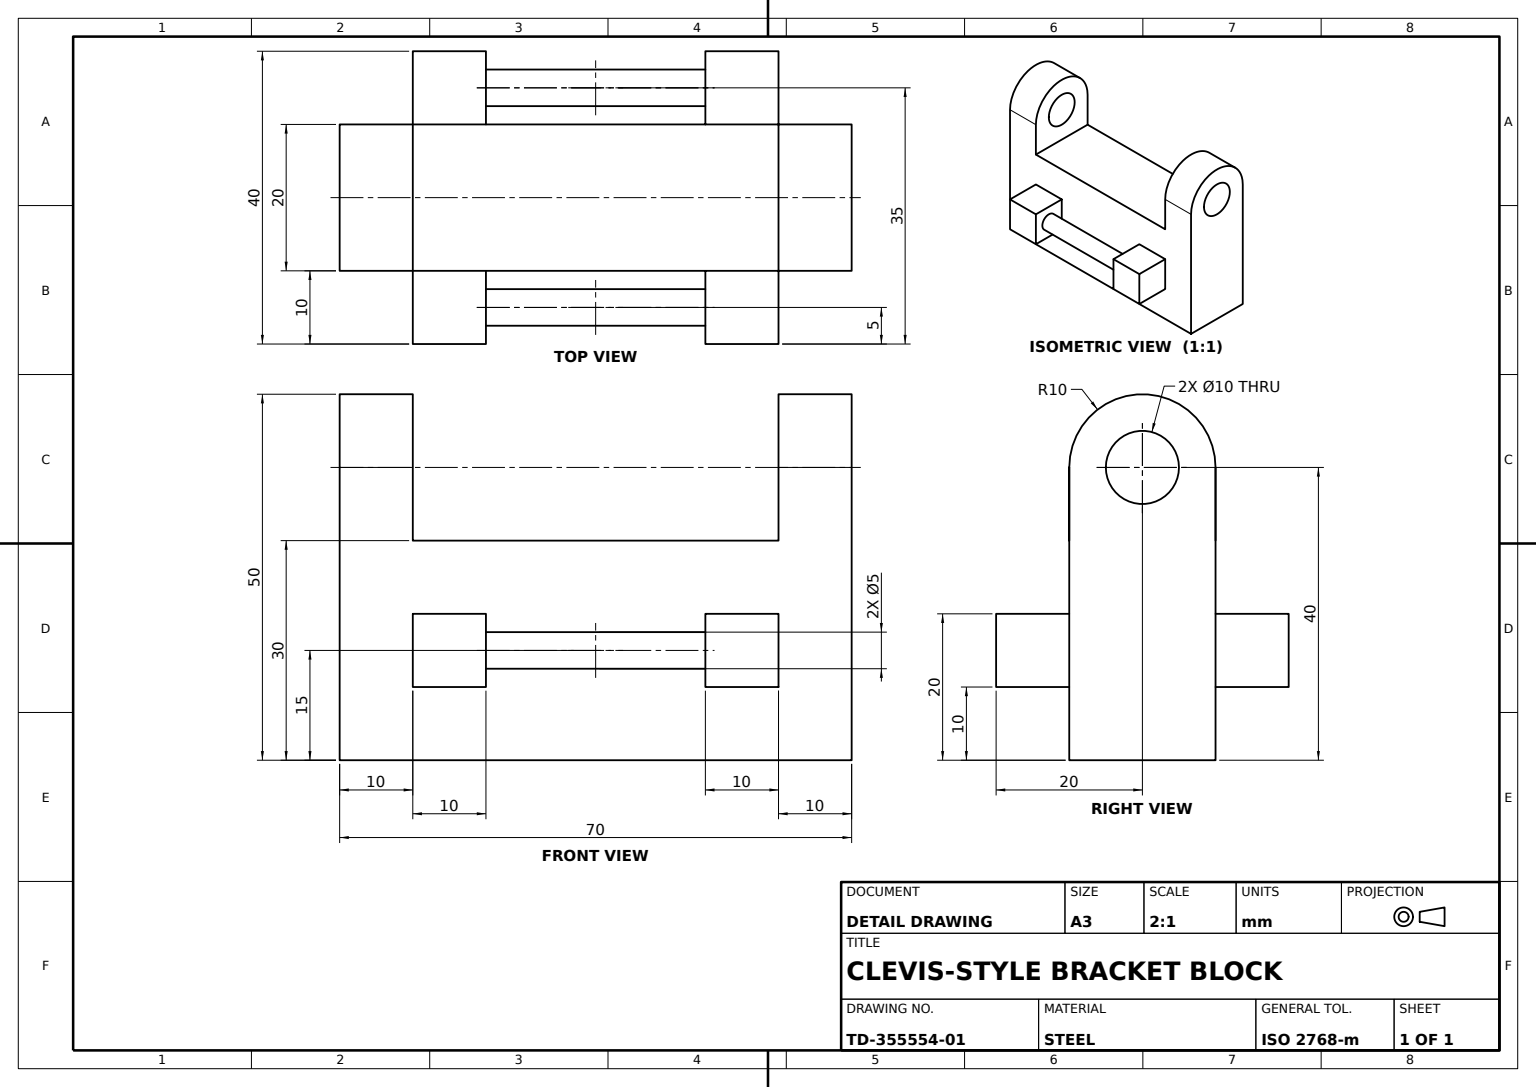
SolidWorks part; units mm, degrees
material "Plain Carbon Steel"
ref_plane "Front Plane" through (0, 0, 0) normal (0, 0, 1) x (1, 0, 0)
ref_plane "Top Plane" through (0, 0, 0) normal (0, 1, 0) x (1, 0, 0)
ref_plane "Right Plane" through (0, 0, 0) normal (1, 0, 0) x (0, 0, -1)
sketch "Base Block Sketch" plane through (0, 0, 0) normal (0, 0, 1) x (1, 0, 0)
  line L0 (0, 0) -> (70, 0)
  line L1 (70, 0) -> (70, 30)
  line L2 (70, 30) -> (0, 30)
  line L3 (0, 30) -> (0, 0)
  dimension "D1" = 70
  dimension "D2" = 30
extrude "Base Block" add sketch "Base Block Sketch" along normal blind 20
ref_plane "Hinge Ear Sketch Plane" through (0, 0, 0) normal (1, 0, 0) x (0, 0, -1)
sketch "Hinge Ear Sketch" plane through (0, 0, 0) normal (1, 0, 0) x (0, 0, -1)
  line L0 (-20, 30) -> (0, 30) construction
  line L1 (-20, 40) -> (-20, 30)
  line L2 (0, 40) -> (0, 30)
  line L3 (0, 30) -> (-20, 30)
  arc A0 (0, 40) -> (-20, 40) centre (-10, 40) ccw
  circle A1 centre (-10, 40) radius 5
  dimension "D1" = 20
  dimension "D2" = 10
  dimension "D3" = 10
extrude "Hinge Ear" add sketch "Hinge Ear Sketch" along normal blind 10
ref_plane "Hinge Ear Mirror Plane" through (35, 0, 0) normal (1, 0, 0) x (0, 0, -1)
mirror "Hinge Ear Mirror" about plane through (35, 0, 0) normal (1, 0, 0) of "Hinge Ear"
sketch "Side Block Sketch" plane through (0, 0, 20) normal (0, 0, 1) x (1, 0, 0)
  line L0 (70, 0) -> (70, 40) construction
  line L1 (50, 20) -> (60, 20)
  line L2 (50, 20) -> (50, 10)
  line L3 (50, 10) -> (60, 10)
  line L4 (60, 20) -> (60, 10)
  line L5 (50, 20) -> (60, 10) construction
  line L6 (50, 10) -> (60, 20) construction
  line L7 (0, 0) -> (70, 0) construction
  point P0 (55, 15)
  dimension "D1" = 10
  dimension "D2" = 10
  dimension "D3" = 10
extrude "Side Block" add sketch "Side Block Sketch" along normal blind 10
sketch "Stop Block Sketch" plane through (0, 0, 20) normal (0, 0, 1) x (1, 0, 0)
  line L0 (0, 40) -> (0, 0) construction
  line L1 (10, 20) -> (20, 20)
  line L2 (10, 20) -> (10, 10)
  line L3 (10, 10) -> (20, 10)
  line L4 (20, 20) -> (20, 10)
  line L5 (0, 0) -> (70, 0) construction
  dimension "D1" = 10
  dimension "D2" = 10
  dimension "D3" = 10
extrude "Stop Block 10mm" add sketch "Stop Block Sketch" along normal blind 10
sketch "Rod Sketch" plane through (20, 0, 0) normal (1, 0, 0) x (0, 0, -1)
  line L0 (-20, 10) -> (-20, 20) construction
  line L1 (-30, 20) -> (-20, 20) construction
  circle A0 centre (-25, 15) radius 2.5
  dimension "D1" = 5
  dimension "D2" = 5
  dimension "D3" = 5
extrude "Rod 30mm" add sketch "Rod Sketch" along normal blind 30
ref_plane "Block and Rod Mirror Plane" through (0, 0, 10) normal (0, 0, 1) x (1, 0, 0)
mirror "Block and Rod Mirror" about plane through (0, 0, 10) normal (0, 0, 1) of "Stop Block 10mm", "Rod 30mm", "Side Block"
